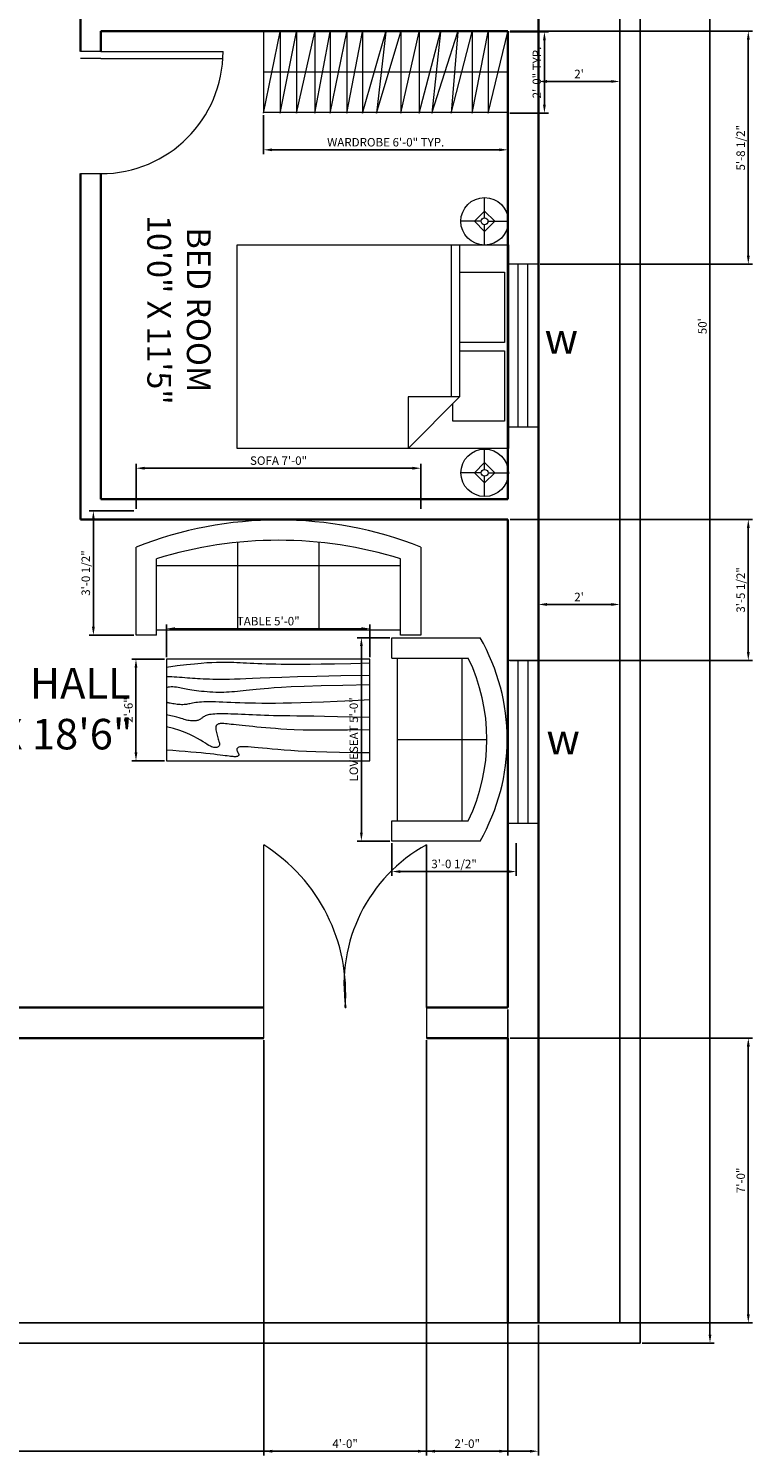
# Model space of a CAD drawing. Units: inches. Extents: x 1879 to 2382, y 1769 to 2461.
# Tile 3 of 5: x 2168 to 2382, y 1769 to 2190. Entities that reach past the tile are written whole.
import ezdxf

# ---------------------------------------------------------------- set-up
doc = ezdxf.new("R2010")
doc.units = ezdxf.units.IN
for name, color, linetype, lineweight in [('A-ANNO-DIMS', 2, 'Continuous', 18), ('A-ANNO-TEXT', 3, 'Continuous', 18), ('A-AREA-IDEN', 7, 'Continuous', 18), ('A-DOOR', 3, 'Continuous', 18), ('A-FLOR-CASE', 8, 'Continuous', 18), ('A-FURN', 9, 'Continuous', 18), ('A-GLAZ', 4, 'Continuous', 18), ('A-WALL', 7, 'Continuous', 35), ('C-PROP', 1, 'Continuous', 25)]:
    doc.layers.add(name, color=color, linetype=linetype, lineweight=lineweight)
doc.styles.get("Standard").update_dxf_attribs({"font": 'arial.ttf'})
doc.dimstyles.new('ISO-25', dxfattribs={"dimtxt": 2.5, "dimasz": 2.5, "dimexe": 1.25, "dimexo": 0.625, "dimtad": 1, "dimlunit": 4, "dimtxsty": 'Standard', "dimcen": 2.5, "dimadec": 0, "dimazin": 0, "dimtfac": 1, "dimtmove": 0, "dimatfit": 3, "dimfxl": 1, "dimarcsym": 0})

# ---------------------------------------------------------------- blocks, each defined once
blk = doc.blocks.new('*D2')
at = {"layer": 'A-ANNO-DIMS', "color": 0, "lineweight": -2, "transparency": 16777216}
for p, q in [((2348.97, 2402.18), (2370.19, 2402.18)), ((2368.94, 2399.68), (2368.94, 1804.68)), ((2348.97, 1802.18), (2370.19, 1802.18))]:
    blk.add_line(p, q, dxfattribs=at)
at = {"layer": 'A-ANNO-DIMS', "color": 0, "transparency": 16777216}
for points in [[(2368.53, 2399.68), (2369.36, 2399.68), (2368.94, 2402.18)], [(2368.53, 1804.68), (2369.36, 1804.68), (2368.94, 1802.18)]]:
    blk.add_solid(points, dxfattribs=at)
at = {"layer": 'Defpoints', "color": 0, "transparency": 16777216}
for p in [(2348.34, 2402.18), (2348.34, 1802.18), (2368.94, 1802.18)]:
    blk.add_point(p, dxfattribs=at)
at = {"layer": 'A-ANNO-DIMS', "color": 0, "transparency": 16777216, "insert": (2367.04, 2102.18), "char_height": 2.5, "attachment_point": 5, "rotation": 90}
blk.add_mtext("50'", dxfattribs=at)
blk = doc.blocks.new('Table - Rectangular Woodgrain 60 x 30 in.')
for p, q in [((0, 0), (0, -30)), ((60, 0), (0, 0)), ((60, -30), (60, 0)), ((0, -30), (60, -30))]:
    blk.add_line(p, q)
for points in [[(0, -2.4), (4.8155, -2.418), (9.0302, -2.4688), (12.709, -2.5477), (15.9167, -2.65), (18.7181, -2.7711), (21.1781, -2.9063), (23.3616, -3.0508), (25.3333, -3.2), (27.1477, -3.3495), (28.8172, -3.4958), (30.3437, -3.636), (31.7291, -3.7667), (32.9756, -3.8849), (34.0849, -3.9875), (35.059, -4.0714), (35.9, -4.1334), (36.6114, -4.1711), (37.2041, -4.1854), (37.6906, -4.1779), (38.0833, -4.15), (38.3948, -4.1034), (38.6375, -4.0396), (38.8239, -3.9602), (38.9666, -3.8667), (39.0764, -3.7608), (39.1573, -3.6448), (39.2116, -3.521), (39.2416, -3.3917), (39.2498, -3.2593), (39.2385, -3.1261), (39.21, -2.9944), (39.1666, -2.8667), (39.111, -2.7447), (39.0468, -2.6281), (38.978, -2.5163), (38.9083, -2.4083), (38.8418, -2.3035), (38.7823, -2.201), (38.7337, -2.1001), (38.7, -2), (38.6844, -1.9003), (38.6875, -1.8021), (38.7094, -1.707), (38.75, -1.6167), (38.8094, -1.5326), (38.8875, -1.4563), (38.9844, -1.3893), (39.1, -1.3333), (39.2351, -1.2896), (39.3937, -1.2583), (39.5804, -1.2396), (39.8, -1.2333), (40.057, -1.2396), (40.3562, -1.2583), (40.7023, -1.2896), (41.1, -1.3333), (41.5547, -1.3895), (42.0755, -1.4573), (42.6721, -1.5361), (43.3542, -1.625), (44.1316, -1.7233), (45.014, -1.8302), (46.0114, -1.9449), (47.1333, -2.0667), (48.3862, -2.1947), (49.7625, -2.3281), (51.2513, -2.4663), (52.8416, -2.6083), (54.5226, -2.7535), (56.2833, -2.9011), (58.1127, -3.0501), (60, -3.2)], [(0, -9.2), (6.5759, -9.0858), (11.9385, -9.0365), (16.2527, -9.0418), (19.6833, -9.0917), (22.3952, -9.1759), (24.5531, -9.2844), (26.322, -9.4069), (27.8666, -9.5333), (29.3241, -9.6553), (30.7203, -9.7719), (32.0532, -9.8837), (33.3208, -9.9917), (34.5213, -10.0965), (35.6526, -10.199), (36.7128, -10.2999), (37.7, -10.4), (38.6129, -10.4996), (39.4531, -10.5969), (40.223, -10.6895), (40.925, -10.775), (41.5613, -10.8512), (42.1344, -10.9156), (42.6465, -10.966), (43.1, -11), (43.4976, -11.0158), (43.8437, -11.0136), (44.143, -10.9942), (44.4, -10.9583), (44.6195, -10.9069), (44.8062, -10.8406), (44.9648, -10.7603), (45.1, -10.6667), (45.2155, -10.5598), (45.3114, -10.4365), (45.3871, -10.2929), (45.4416, -10.125), (45.4743, -9.929), (45.4844, -9.7011), (45.4709, -9.4371), (45.4333, -9.1333), (45.3716, -8.7883), (45.2896, -8.4104), (45.1919, -8.0107), (45.0833, -7.6), (44.9685, -7.1893), (44.8521, -6.7896), (44.7388, -6.4117), (44.6333, -6.0667), (44.54, -5.7628), (44.4614, -5.4979), (44.4001, -5.2675), (44.3583, -5.0667), (44.3384, -4.8909), (44.3427, -4.7354), (44.3736, -4.5956), (44.4333, -4.4667), (44.5236, -4.3453), (44.6427, -4.2333), (44.7884, -4.1339), (44.9583, -4.05), (45.1501, -3.9849), (45.3614, -3.9417), (45.59, -3.9234), (45.8333, -3.9333), (46.0915, -3.9749), (46.3734, -4.0531), (46.6906, -4.1736), (47.0542, -4.3417), (47.4756, -4.5629), (47.9661, -4.8427), (48.5372, -5.1866), (49.2, -5.6), (49.9676, -6.0844), (50.8594, -6.625), (51.8965, -7.2031), (53.1, -7.8), (54.491, -8.3969), (56.0906, -8.975), (57.9199, -9.5156), (60, -10)], [(0, -12.8), (5.1847, -12.9322), (9.6213, -13.0323), (13.3963, -13.1059), (16.5958, -13.1583), (19.3063, -13.1952), (21.614, -13.2219), (23.6054, -13.2439), (25.3666, -13.2667), (26.9728, -13.2947), (28.4531, -13.3281), (29.8256, -13.3663), (31.1083, -13.4083), (32.3191, -13.4535), (33.476, -13.501), (34.597, -13.5501), (35.7, -13.6), (36.7984, -13.6497), (37.8875, -13.6979), (38.9578, -13.743), (40, -13.7833), (41.0047, -13.8174), (41.9625, -13.8438), (42.864, -13.8607), (43.7, -13.8667), (44.4631, -13.8604), (45.1552, -13.8417), (45.7801, -13.8104), (46.3416, -13.7667), (46.8439, -13.7104), (47.2906, -13.6417), (47.6858, -13.5604), (48.0333, -13.4667), (48.3375, -13.3608), (48.6042, -13.2448), (48.8396, -13.121), (49.05, -12.9917), (49.2417, -12.8593), (49.4208, -12.7261), (49.5937, -12.5944), (49.7667, -12.4667), (49.9452, -12.3451), (50.1323, -12.2313), (50.3303, -12.1268), (50.5416, -12.0333), (50.7686, -11.9524), (51.0135, -11.8854), (51.2788, -11.8341), (51.5666, -11.8), (51.8785, -11.7843), (52.2116, -11.7865), (52.562, -11.8059), (52.926, -11.8417), (53.2998, -11.8931), (53.6795, -11.9594), (54.0614, -12.0397), (54.4416, -12.1333), (54.8223, -12.2401), (55.2293, -12.3625), (55.6942, -12.5037), (56.2489, -12.6667), (56.9251, -12.8547), (57.7545, -13.0708), (58.7689, -13.3182), (60, -13.6)], [(0, -18), (5.124, -17.7273), (9.6609, -17.5057), (13.6705, -17.3303), (17.2125, -17.1958), (20.3467, -17.0973), (23.1328, -17.0297), (25.6307, -16.9878), (27.9, -16.9667), (29.9928, -16.9617), (31.9302, -16.9703), (33.7254, -16.9907), (35.3917, -17.0208), (36.9423, -17.0588), (38.3906, -17.1026), (39.7499, -17.1503), (41.0333, -17.2), (42.2519, -17.2496), (43.4073, -17.2969), (44.4986, -17.3395), (45.525, -17.375), (46.4858, -17.4012), (47.3802, -17.4156), (48.2074, -17.416), (48.9667, -17.4), (49.6583, -17.3662), (50.2872, -17.3167), (50.8595, -17.2547), (51.3812, -17.1833), (51.8584, -17.1057), (52.2971, -17.025), (52.7034, -16.9443), (53.0833, -16.8667), (53.443, -16.7951), (53.789, -16.7313), (54.128, -16.6768), (54.4666, -16.6334), (54.8115, -16.6024), (55.1693, -16.5854), (55.5465, -16.5841), (55.95, -16.6), (56.3828, -16.6337), (56.8346, -16.6823), (57.2915, -16.7418), (57.7396, -16.8084), (58.165, -16.878), (58.5539, -16.9469), (58.8924, -17.0111), (59.1666, -17.0667), (59.3679, -17.1107), (59.5078, -17.1438), (59.6032, -17.1675), (59.6708, -17.1833), (59.7275, -17.193), (59.7901, -17.1979), (59.8753, -17.1998), (60, -17.2)], [(0, -22.4), (8.0098, -22.2501), (14.4094, -22.1011), (19.4168, -21.9535), (23.25, -21.8083), (26.1269, -21.6663), (28.2656, -21.5281), (29.884, -21.3947), (31.2, -21.2667), (32.3967, -21.1448), (33.5172, -21.0292), (34.5697, -20.9198), (35.5625, -20.8167), (36.5037, -20.7198), (37.4015, -20.6292), (38.2642, -20.5448), (39.1, -20.4667), (39.9164, -20.3951), (40.7187, -20.3313), (41.5117, -20.2768), (42.3, -20.2333), (43.0883, -20.2024), (43.8812, -20.1854), (44.6836, -20.1841), (45.5, -20.2), (46.3328, -20.234), (47.1747, -20.2844), (48.0163, -20.3488), (48.8479, -20.425), (49.66, -20.5106), (50.4429, -20.6031), (51.1872, -20.7004), (51.8833, -20.8), (52.5246, -20.8999), (53.1166, -20.9995), (53.6681, -21.0983), (54.1875, -21.1958), (54.6834, -21.2919), (55.1646, -21.3859), (55.6394, -21.4777), (56.1167, -21.5667), (56.6028, -21.6515), (57.0961, -21.7266), (57.5929, -21.7852), (58.0896, -21.8208), (58.5823, -21.8268), (59.0674, -21.7964), (59.5412, -21.723), (60, -21.6)], [(0, -25.2), (8.6355, -25.0504), (15.7026, -24.9031), (21.4049, -24.7606), (25.9458, -24.625), (29.529, -24.4988), (32.3578, -24.3844), (34.6359, -24.284), (36.5667, -24.2), (38.3213, -24.1341), (39.9417, -24.0854), (41.437, -24.0523), (42.8167, -24.0333), (44.0901, -24.0268), (45.2667, -24.0313), (46.3557, -24.0451), (47.3667, -24.0667), (48.309, -24.0947), (49.1928, -24.1287), (50.0284, -24.168), (50.826, -24.2125), (51.5959, -24.2617), (52.3483, -24.3151), (53.0935, -24.3725), (53.8417, -24.4334), (54.6009, -24.497), (55.3699, -24.561), (56.1454, -24.6226), (56.9239, -24.6792), (57.7021, -24.7279), (58.4764, -24.7662), (59.2435, -24.7911), (60, -24.8)], [(0, -28.8), (5.6867, -28.6681), (10.45, -28.5698), (14.407, -28.5012), (17.675, -28.4584), (20.3711, -28.4374), (22.6125, -28.4344), (24.5164, -28.4455), (26.2, -28.4667), (27.762, -28.4947), (29.2276, -28.5281), (30.6033, -28.5663), (31.8958, -28.6084), (33.1118, -28.6535), (34.2578, -28.7011), (35.3405, -28.7501), (36.3666, -28.8), (37.3443, -28.8497), (38.288, -28.8974), (39.2137, -28.9412), (40.1375, -28.9792), (41.0753, -29.0093), (42.0432, -29.0297), (43.0572, -29.0384), (44.1333, -29.0333), (45.2936, -29.0114), (46.5843, -28.9641), (48.0579, -28.8816), (49.7666, -28.7542), (51.7629, -28.5721), (54.0989, -28.3255), (56.8272, -28.0048), (60, -27.6)]]:
    blk.add_lwpolyline(points)
blk = doc.blocks.new('Sofa - Roundback 7 ft.')
for p, q in [((-12.00002, -32.4421), (-12.00003, -6.5971)), ((11.99997, -32.4421), (11.99998, -6.5971)), ((-36.000027, -34), (-36.000027, -11.4696)), ((35.99998, -34), (35.99998, -11.4696)), ((-35.999844, -13.3819), (35.9998, -13.3819)), ((-36.000027, -32.4421), (35.99998, -32.4421))]:
    blk.add_line(p, q)
for points in [[(-36.000027, -34), (-42.000027, -34), (-42.000027, -8)], [(41.99998, -8), (41.99998, -34), (35.99998, -34)]]:
    blk.add_lwpolyline(points)
for centre, radius, start, end in [((0, -114.25), 114.25, 68.43141, 111.5686), ((-0.00001, -127.1968), 121.1968, 72.72033, 107.2797)]:
    blk.add_arc(centre, radius, start, end)
blk = doc.blocks.new('Sofa - Roundback Loveseat 5 ft.')
for p, q in [((0, -32.44198), (0, -5.99998)), ((-24, -33.99998), (-24, -11.46958)), ((24.00004, -33.99998), (24.00004, -11.46958)), ((-23.9998, -13.38178), (23.99986, -13.38178)), ((-24, -32.44198), (24.00004, -32.44198))]:
    blk.add_line(p, q)
for points in [[(-24, -33.99998), (-30, -33.99998), (-30, -7.99998)], [(30.00004, -7.99998), (30.00004, -33.99998), (24.00004, -33.99998)]]:
    blk.add_lwpolyline(points)
for centre, radius, start, end in [((0, -60.24998), 60.24998, 60.13715, 119.8628), ((0, -61.38438), 55.38444, 64.32083, 115.6792)]:
    blk.add_arc(centre, radius, start, end)
blk = doc.blocks.new('Bed - Queen')
for p, q in [((0, -80.00003), (0, 0)), ((0, 0), (59.99999, 0)), ((59.99999, 0), (59.99999, -80.00003)), ((7.99999, -1.2), (28.79998, -1.2)), ((7.99999, -14.4), (7.99999, -1.2)), ((28.79998, -1.2), (28.79998, -14.4)), ((31.19999, -1.2), (51.99999, -1.2)), ((31.19999, -14.4), (31.19999, -1.2)), ((51.99999, -1.2), (51.99999, -16.4)), ((0, -14.4), (44.8, -14.4)), ((44.8, -16.8), (0, -16.8)), ((59.99999, -29.6), (44.8, -14.4)), ((44.8, -14.4), (44.8, -29.6)), ((51.99999, -16.4), (46.79936, -16.4)), ((44.8, -29.6), (59.99999, -29.6)), ((59.99999, -80.00003), (0, -80.00003))]:
    blk.add_line(p, q)
blk = doc.blocks.new('Lamp - Table')
for p, q in [((0, 7), (0, 1)), ((-1, 0), (-7, 0)), ((0, 3), (-3, 0)), ((-3, 0), (0, -3)), ((3, 0), (0, 3)), ((0, -3), (3, 0)), ((1, 0), (7, 0)), ((0, -1), (0, -7))]:
    blk.add_line(p, q)
for radius in [7, 1]:
    blk.add_circle((0, 0), radius)
blk = doc.blocks.new('*D17')
at = {"layer": 'A-ANNO-DIMS', "color": 0, "lineweight": -2, "transparency": 16777216}
for p, q in [((2318.34, 2188.56), (2318.34, 2173.13)), ((2342.34, 2188.56), (2342.34, 2173.13)), ((2320.84, 2174.38), (2339.84, 2174.38))]:
    blk.add_line(p, q, dxfattribs=at)
at = {"layer": 'A-ANNO-DIMS', "color": 0, "transparency": 16777216}
for points in [[(2320.84, 2174.8), (2320.84, 2173.97), (2318.34, 2174.38)], [(2339.84, 2174.8), (2339.84, 2173.97), (2342.34, 2174.38)]]:
    blk.add_solid(points, dxfattribs=at)
at = {"layer": 'Defpoints', "color": 0, "transparency": 16777216}
for p in [(2318.34, 2189.18), (2342.34, 2189.18), (2342.34, 2174.38)]:
    blk.add_point(p, dxfattribs=at)
at = {"layer": 'A-ANNO-DIMS', "color": 0, "transparency": 16777216, "insert": (2330.34, 2176.26), "char_height": 2.5, "attachment_point": 5}
blk.add_mtext("2'", dxfattribs=at)
blk = doc.blocks.new('*D18')
at = {"layer": 'A-ANNO-DIMS', "color": 0, "lineweight": -2, "transparency": 16777216}
for p, q in [((2318.34, 2020.71), (2318.34, 2021.34)), ((2342.34, 2020.71), (2342.34, 2021.34)), ((2339.84, 2020.09), (2320.84, 2020.09))]:
    blk.add_line(p, q, dxfattribs=at)
at = {"layer": 'A-ANNO-DIMS', "color": 0, "transparency": 16777216}
for points in [[(2320.84, 2020.51), (2320.84, 2019.67), (2318.34, 2020.09)], [(2339.84, 2020.51), (2339.84, 2019.67), (2342.34, 2020.09)]]:
    blk.add_solid(points, dxfattribs=at)
at = {"layer": 'Defpoints', "color": 0, "transparency": 16777216}
for p in [(2318.34, 2020.09), (2318.34, 2020.09), (2342.34, 2020.09)]:
    blk.add_point(p, dxfattribs=at)
at = {"layer": 'A-ANNO-DIMS', "color": 0, "transparency": 16777216, "insert": (2330.34, 2021.97), "char_height": 2.5, "attachment_point": 5}
blk.add_mtext("2'", dxfattribs=at)
blk = doc.blocks.new('WN-48x9')
for p, q in [((0, 48), (0, 0)), ((9, 48), (0, 48)), ((3, 48), (3, 0)), ((6, 0), (6, 48)), ((9, 0), (9, 48)), ((0, 0), (9, 0))]:
    blk.add_line(p, q)
blk = doc.blocks.new('DR-SWING-36')
for p, q in [((42, 36), (36, 36)), ((36, 2), (0, 2)), ((36, 0), (0, 0)), ((36, 2), (42, 2)), ((36, 0), (42, 0))]:
    blk.add_line(p, q)
blk.add_arc((36, 0), 36, 90, 180)
blk = doc.blocks.new('WARDROBE-HANGERS-72')
for p, q in [((0, 0), (4.89, 24)), ((4.89, 24), (4.89, 0)), ((4.89, 0), (9.67, 24)), ((9.67, 24), (9.67, 0)), ((9.67, 0), (15.08, 24)), ((15.08, 24), (15.08, 0)), ((15.08, 0), (19.6, 24)), ((19.6, 24), (19.6, 0)), ((19.6, 0), (24.51, 24)), ((24.51, 24), (24.51, 0)), ((24.51, 0), (29.16, 24)), ((29.16, 24), (29.16, 0)), ((29.16, 0), (36, 24)), ((36, 24), (33.31, 0)), ((33.31, 0), (40.47, 24)), ((40.47, 24), (40.47, 0)), ((40.47, 0), (45.88, 24)), ((45.88, 24), (45.88, 0)), ((45.88, 0), (52.17, 24)), ((52.17, 24), (49.65, 0)), ((49.65, 0), (57.32, 24)), ((57.32, 24), (55.31, 0)), ((55.31, 0), (61.47, 24)), ((61.47, 24), (61.47, 0)), ((61.47, 0), (66.25, 24)), ((66.25, 24), (66.25, 0)), ((66.25, 0), (72, 24))]:
    blk.add_line(p, q)
blk = doc.blocks.new('*D37')
at = {"layer": 'A-ANNO-DIMS', "color": 0, "lineweight": -2, "transparency": 16777216}
for p, q in [((2237.31, 2164.39), (2237.31, 2152.97)), ((2309.31, 2164.39), (2309.31, 2152.97)), ((2239.81, 2154.22), (2306.81, 2154.22))]:
    blk.add_line(p, q, dxfattribs=at)
at = {"layer": 'A-ANNO-DIMS', "color": 0, "transparency": 16777216}
for points in [[(2239.81, 2154.63), (2239.81, 2153.8), (2237.31, 2154.22)], [(2306.81, 2154.63), (2306.81, 2153.8), (2309.31, 2154.22)]]:
    blk.add_solid(points, dxfattribs=at)
at = {"layer": 'Defpoints', "color": 0, "transparency": 16777216}
for p in [(2237.31, 2165.02), (2309.31, 2165.02), (2309.31, 2154.22)]:
    blk.add_point(p, dxfattribs=at)
at = {"layer": 'A-ANNO-DIMS', "color": 0, "transparency": 16777216, "insert": (2273.31, 2156.13), "char_height": 2.5, "attachment_point": 5}
blk.add_mtext('WARDROBE 6\'-0" TYP.', dxfattribs=at)
blk = doc.blocks.new('*D38')
at = {"layer": 'A-ANNO-DIMS', "color": 0, "lineweight": -2, "transparency": 16777216}
for p, q in [((2309.93, 2189.02), (2321.36, 2189.02)), ((2320.11, 2167.52), (2320.11, 2186.52)), ((2309.93, 2165.02), (2321.36, 2165.02))]:
    blk.add_line(p, q, dxfattribs=at)
at = {"layer": 'A-ANNO-DIMS', "color": 0, "transparency": 16777216}
for points in [[(2319.69, 2186.52), (2320.53, 2186.52), (2320.11, 2189.02)], [(2319.69, 2167.52), (2320.53, 2167.52), (2320.11, 2165.02)]]:
    blk.add_solid(points, dxfattribs=at)
at = {"layer": 'Defpoints', "color": 0, "transparency": 16777216}
for p in [(2309.31, 2189.02), (2320.11, 2189.02), (2309.31, 2165.02)]:
    blk.add_point(p, dxfattribs=at)
at = {"layer": 'A-ANNO-DIMS', "color": 0, "transparency": 16777216, "insert": (2318.21, 2177.02), "char_height": 2.5, "attachment_point": 5, "rotation": 90}
blk.add_mtext('2\'-0" TYP.', dxfattribs=at)
blk = doc.blocks.new('*D47')
at = {"layer": 'A-ANNO-DIMS', "color": 0, "lineweight": -2, "transparency": 16777216}
for p, q in [((2199.71, 2048.3), (2199.71, 2061.53)), ((2202.21, 2060.28), (2281.21, 2060.28)), ((2283.71, 2048.3), (2283.71, 2061.53))]:
    blk.add_line(p, q, dxfattribs=at)
at = {"layer": 'A-ANNO-DIMS', "color": 0, "transparency": 16777216}
for points in [[(2202.21, 2060.7), (2202.21, 2059.86), (2199.71, 2060.28)], [(2281.21, 2060.7), (2281.21, 2059.86), (2283.71, 2060.28)]]:
    blk.add_solid(points, dxfattribs=at)
at = {"layer": 'Defpoints', "color": 0, "transparency": 16777216}
for p in [(2283.71, 2060.28), (2199.71, 2047.68), (2283.71, 2047.68)]:
    blk.add_point(p, dxfattribs=at)
at = {"layer": 'A-ANNO-DIMS', "color": 0, "transparency": 16777216, "insert": (2241.71, 2062.2), "char_height": 2.5, "attachment_point": 5}
blk.add_mtext('SOFA 7\'-0"', dxfattribs=at)
blk = doc.blocks.new('*D48')
at = {"layer": 'A-ANNO-DIMS', "color": 0, "lineweight": -2, "transparency": 16777216}
for p, q in [((2199.08, 2047.68), (2185.86, 2047.68)), ((2187.11, 2013.51), (2187.11, 2045.18)), ((2199.08, 2011.01), (2185.86, 2011.01))]:
    blk.add_line(p, q, dxfattribs=at)
at = {"layer": 'A-ANNO-DIMS', "color": 0, "transparency": 16777216}
for points in [[(2186.69, 2045.18), (2187.52, 2045.18), (2187.11, 2047.68)], [(2186.69, 2013.51), (2187.52, 2013.51), (2187.11, 2011.01)]]:
    blk.add_solid(points, dxfattribs=at)
at = {"layer": 'Defpoints', "color": 0, "transparency": 16777216}
for p in [(2187.11, 2047.68), (2199.71, 2047.68), (2199.71, 2011.01)]:
    blk.add_point(p, dxfattribs=at)
at = {"layer": 'A-ANNO-DIMS', "color": 0, "transparency": 16777216, "insert": (2185.19, 2029.35), "char_height": 2.5, "attachment_point": 5, "rotation": 90}
blk.add_mtext('3\'-0 1/2"', dxfattribs=at)
blk = doc.blocks.new('*D49')
at = {"layer": 'A-ANNO-DIMS', "color": 0, "lineweight": -2, "transparency": 16777216}
for p, q in [((2274.52, 2010.29), (2264.89, 2010.29)), ((2266.14, 2007.79), (2266.14, 1952.79)), ((2274.52, 1950.29), (2264.89, 1950.29))]:
    blk.add_line(p, q, dxfattribs=at)
at = {"layer": 'A-ANNO-DIMS', "color": 0, "transparency": 16777216}
for points in [[(2265.73, 2007.79), (2266.56, 2007.79), (2266.14, 2010.29)], [(2265.73, 1952.79), (2266.56, 1952.79), (2266.14, 1950.29)]]:
    blk.add_solid(points, dxfattribs=at)
at = {"layer": 'Defpoints', "color": 0, "transparency": 16777216}
for p in [(2275.14, 2010.29), (2266.14, 1950.29), (2275.14, 1950.29)]:
    blk.add_point(p, dxfattribs=at)
at = {"layer": 'A-ANNO-DIMS', "color": 0, "transparency": 16777216, "insert": (2264.22, 1980.29), "char_height": 2.5, "attachment_point": 5, "rotation": 90}
blk.add_mtext('LOVESEAT 5\'-0"', dxfattribs=at)
blk = doc.blocks.new('*D50')
at = {"layer": 'A-ANNO-DIMS', "color": 0, "lineweight": -2, "transparency": 16777216}
for p, q in [((2275.14, 1949.66), (2275.14, 1940.04)), ((2311.81, 1949.66), (2311.81, 1940.04)), ((2277.64, 1941.29), (2309.31, 1941.29))]:
    blk.add_line(p, q, dxfattribs=at)
at = {"layer": 'A-ANNO-DIMS', "color": 0, "transparency": 16777216}
for points in [[(2277.64, 1941.7), (2277.64, 1940.87), (2275.14, 1941.29)], [(2309.31, 1941.7), (2309.31, 1940.87), (2311.81, 1941.29)]]:
    blk.add_solid(points, dxfattribs=at)
at = {"layer": 'Defpoints', "color": 0, "transparency": 16777216}
for p in [(2275.14, 1950.29), (2311.81, 1950.29), (2311.81, 1941.29)]:
    blk.add_point(p, dxfattribs=at)
at = {"layer": 'A-ANNO-DIMS', "color": 0, "transparency": 16777216, "insert": (2293.48, 1943.21), "char_height": 2.5, "attachment_point": 5}
blk.add_mtext('3\'-0 1/2"', dxfattribs=at)
blk = doc.blocks.new('*D51')
at = {"layer": 'A-ANNO-DIMS', "color": 0, "lineweight": -2, "transparency": 16777216}
for p, q in [((2208.67, 2004.57), (2208.67, 2014.19)), ((2266.17, 2012.94), (2211.17, 2012.94)), ((2268.67, 2004.57), (2268.67, 2014.19))]:
    blk.add_line(p, q, dxfattribs=at)
at = {"layer": 'A-ANNO-DIMS', "color": 0, "transparency": 16777216}
for points in [[(2211.17, 2013.36), (2211.17, 2012.52), (2208.67, 2012.94)], [(2266.17, 2013.36), (2266.17, 2012.52), (2268.67, 2012.94)]]:
    blk.add_solid(points, dxfattribs=at)
at = {"layer": 'Defpoints', "color": 0, "transparency": 16777216}
for p in [(2208.67, 2012.94), (2208.67, 2003.94), (2268.67, 2003.94)]:
    blk.add_point(p, dxfattribs=at)
at = {"layer": 'A-ANNO-DIMS', "color": 0, "transparency": 16777216, "insert": (2238.67, 2014.84), "char_height": 2.5, "attachment_point": 5}
blk.add_mtext('TABLE 5\'-0"', dxfattribs=at)
blk = doc.blocks.new('*D52')
at = {"layer": 'A-ANNO-DIMS', "color": 0, "lineweight": -2, "transparency": 16777216}
for p, q in [((2208.04, 2003.94), (2198.42, 2003.94)), ((2199.67, 2001.44), (2199.67, 1976.44)), ((2208.04, 1973.94), (2198.42, 1973.94))]:
    blk.add_line(p, q, dxfattribs=at)
at = {"layer": 'A-ANNO-DIMS', "color": 0, "transparency": 16777216}
for points in [[(2199.25, 2001.44), (2200.08, 2001.44), (2199.67, 2003.94)], [(2199.25, 1976.44), (2200.08, 1976.44), (2199.67, 1973.94)]]:
    blk.add_solid(points, dxfattribs=at)
at = {"layer": 'Defpoints', "color": 0, "transparency": 16777216}
for p in [(2208.67, 2003.94), (2199.67, 1973.94), (2208.67, 1973.94)]:
    blk.add_point(p, dxfattribs=at)
at = {"layer": 'A-ANNO-DIMS', "color": 0, "transparency": 16777216, "insert": (2197.77, 1988.94), "char_height": 2.5, "attachment_point": 5, "rotation": 90}
blk.add_mtext('2\'-6"', dxfattribs=at)
blk = doc.blocks.new('*D55')
at = {"layer": 'A-ANNO-DIMS', "color": 0, "lineweight": -2, "transparency": 16777216}
for p, q in [((1946.34, 1807.56), (1946.34, 1769.03)), ((2318.34, 1807.56), (2318.34, 1769.03)), ((1948.84, 1770.28), (2315.84, 1770.28))]:
    blk.add_line(p, q, dxfattribs=at)
at = {"layer": 'A-ANNO-DIMS', "color": 0, "transparency": 16777216}
for points in [[(1948.84, 1770.7), (1948.84, 1769.86), (1946.34, 1770.28)], [(2315.84, 1770.7), (2315.84, 1769.86), (2318.34, 1770.28)]]:
    blk.add_solid(points, dxfattribs=at)
at = {"layer": 'Defpoints', "color": 0, "transparency": 16777216}
for p in [(1946.34, 1808.18), (2318.34, 1808.18), (2318.34, 1770.28)]:
    blk.add_point(p, dxfattribs=at)
at = {"layer": 'A-ANNO-DIMS', "color": 0, "transparency": 16777216, "insert": (2132.34, 1772.18), "char_height": 2.5, "attachment_point": 5}
blk.add_mtext('31\'-0"', dxfattribs=at)
blk = doc.blocks.new('*D57')
at = {"layer": 'A-ANNO-DIMS', "color": 0, "lineweight": -2, "transparency": 16777216}
for p, q in [((2309.97, 1892.18), (2381.49, 1892.18)), ((2380.24, 1889.68), (2380.24, 1810.68)), ((2309.97, 1808.18), (2381.49, 1808.18))]:
    blk.add_line(p, q, dxfattribs=at)
at = {"layer": 'A-ANNO-DIMS', "color": 0, "transparency": 16777216}
for points in [[(2379.82, 1889.68), (2380.66, 1889.68), (2380.24, 1892.18)], [(2379.82, 1810.68), (2380.66, 1810.68), (2380.24, 1808.18)]]:
    blk.add_solid(points, dxfattribs=at)
at = {"layer": 'Defpoints', "color": 0, "transparency": 16777216}
for p in [(2309.34, 1892.18), (2309.34, 1808.18), (2380.24, 1808.18)]:
    blk.add_point(p, dxfattribs=at)
at = {"layer": 'A-ANNO-DIMS', "color": 0, "transparency": 16777216, "insert": (2378.34, 1850.18), "char_height": 2.5, "attachment_point": 5, "rotation": 90}
blk.add_mtext('7\'-0"', dxfattribs=at)
blk = doc.blocks.new('*D59')
at = {"layer": 'A-ANNO-DIMS', "color": 0, "lineweight": -2, "transparency": 16777216}
for p, q in [((2237.34, 1891.56), (2237.34, 1769.03)), ((2285.34, 1891.56), (2285.34, 1769.03)), ((2239.84, 1770.28), (2282.84, 1770.28))]:
    blk.add_line(p, q, dxfattribs=at)
at = {"layer": 'A-ANNO-DIMS', "color": 0, "transparency": 16777216}
for points in [[(2239.84, 1770.7), (2239.84, 1769.86), (2237.34, 1770.28)], [(2282.84, 1770.7), (2282.84, 1769.86), (2285.34, 1770.28)]]:
    blk.add_solid(points, dxfattribs=at)
at = {"layer": 'Defpoints', "color": 0, "transparency": 16777216}
for p in [(2237.34, 1892.18), (2285.34, 1892.18), (2285.34, 1770.28)]:
    blk.add_point(p, dxfattribs=at)
at = {"layer": 'A-ANNO-DIMS', "color": 0, "transparency": 16777216, "insert": (2261.34, 1772.18), "char_height": 2.5, "attachment_point": 5}
blk.add_mtext('4\'-0"', dxfattribs=at)
blk = doc.blocks.new('*D60')
at = {"layer": 'A-ANNO-DIMS', "color": 0, "lineweight": -2, "transparency": 16777216}
for p, q in [((2309.34, 1900.56), (2309.34, 1769.03)), ((2285.34, 1891.56), (2285.34, 1769.03)), ((2287.84, 1770.28), (2306.84, 1770.28))]:
    blk.add_line(p, q, dxfattribs=at)
at = {"layer": 'A-ANNO-DIMS', "color": 0, "transparency": 16777216}
for points in [[(2287.84, 1770.7), (2287.84, 1769.86), (2285.34, 1770.28)], [(2306.84, 1770.7), (2306.84, 1769.86), (2309.34, 1770.28)]]:
    blk.add_solid(points, dxfattribs=at)
at = {"layer": 'Defpoints', "color": 0, "transparency": 16777216}
for p in [(2309.34, 1901.18), (2285.34, 1892.18), (2309.34, 1770.28)]:
    blk.add_point(p, dxfattribs=at)
at = {"layer": 'A-ANNO-DIMS', "color": 0, "transparency": 16777216, "insert": (2297.34, 1772.18), "char_height": 2.5, "attachment_point": 5}
blk.add_mtext('2\'-0"', dxfattribs=at)
blk = doc.blocks.new('*D69')
at = {"layer": 'A-ANNO-DIMS', "color": 0, "lineweight": -2, "transparency": 16777216}
for p, q in [((2309.97, 2189.18), (2381.49, 2189.18)), ((2380.24, 2122.96), (2380.24, 2186.68)), ((2318.89, 2120.46), (2381.49, 2120.46))]:
    blk.add_line(p, q, dxfattribs=at)
at = {"layer": 'A-ANNO-DIMS', "color": 0, "transparency": 16777216}
for points in [[(2379.82, 2186.68), (2380.66, 2186.68), (2380.24, 2189.18)], [(2379.82, 2122.96), (2380.66, 2122.96), (2380.24, 2120.46)]]:
    blk.add_solid(points, dxfattribs=at)
at = {"layer": 'Defpoints', "color": 0, "transparency": 16777216}
for p in [(2309.34, 2189.18), (2380.24, 2189.18), (2318.27, 2120.46)]:
    blk.add_point(p, dxfattribs=at)
at = {"layer": 'A-ANNO-DIMS', "color": 0, "transparency": 16777216, "insert": (2378.32, 2154.82), "char_height": 2.5, "attachment_point": 5, "rotation": 90}
blk.add_mtext('5\'-8 1/2"', dxfattribs=at)
blk = doc.blocks.new('*D76')
at = {"layer": 'A-ANNO-DIMS', "color": 0, "lineweight": -2, "transparency": 16777216}
for p, q in [((2309.97, 2045.18), (2381.49, 2045.18)), ((2380.24, 2042.68), (2380.24, 2006.07)), ((2309.94, 2003.57), (2381.49, 2003.57))]:
    blk.add_line(p, q, dxfattribs=at)
at = {"layer": 'A-ANNO-DIMS', "color": 0, "transparency": 16777216}
for points in [[(2379.82, 2042.68), (2380.66, 2042.68), (2380.24, 2045.18)], [(2379.82, 2006.07), (2380.66, 2006.07), (2380.24, 2003.57)]]:
    blk.add_solid(points, dxfattribs=at)
at = {"layer": 'Defpoints', "color": 0, "transparency": 16777216}
for p in [(2309.34, 2045.18), (2309.31, 2003.57), (2380.24, 2003.57)]:
    blk.add_point(p, dxfattribs=at)
at = {"layer": 'A-ANNO-DIMS', "color": 0, "transparency": 16777216, "insert": (2378.32, 2024.38), "char_height": 2.5, "attachment_point": 5, "rotation": 90}
blk.add_mtext('3\'-5 1/2"', dxfattribs=at)

msp = doc.modelspace()

# ---------------------------------------------------------------- linework, layer by layer
at = {"layer": 'A-DOOR'}
for p, q in [((2237.341, 1901.18), (2237.341, 1949.18)), ((2285.341, 1901.18), (2285.341, 1949.18)), ((2285.341, 1949.18), (2285.341, 1901.18)), ((2237.341, 1892.18), (2237.341, 1901.18)), ((2261.341, 1901.18), (2261.507, 1901.18)), ((2261.507, 1901.18), (2261.341, 1901.18)), ((2261.507, 1901.18), (2261.341, 1901.18)), ((2285.341, 1901.18), (2285.341, 1892.18))]:
    msp.add_line(p, q, dxfattribs=at)
for centre, radius, start, end in [((2209.623, 1905.321), 51.883, 355.42213, 57.70797), ((2307.924, 1908.049), 46.923, 118.76884, 188.41761)]:
    msp.add_arc(centre, radius, start, end, dxfattribs=at)
at = {"layer": 'A-FLOR-CASE'}
for p, q in [((2237.341, 2165.18), (2237.341, 2189.18)), ((2309.341, 2189.18), (2309.341, 2165.18)), ((2237.341, 2177.18), (2309.341, 2177.18)), ((2309.341, 2165.18), (2237.341, 2165.18))]:
    msp.add_line(p, q, dxfattribs=at)
at = {"layer": 'A-WALL'}
for p, q in [((2318.341, 2369.18), (2318.341, 1808.18)), ((2183.341, 2205.18), (2183.341, 2189.18)), ((2183.341, 2189.18), (2183.341, 2183.18)), ((2189.341, 2189.18), (2309.341, 2189.18)), ((2189.341, 2189.18), (2189.341, 2183.18)), ((2189.341, 2189.18), (2189.341, 2183.18)), ((2309.341, 2189.18), (2309.341, 2051.18)), ((2183.341, 2147.18), (2183.341, 2045.18)), ((2189.341, 2147.18), (2189.341, 2051.18)), ((2189.341, 2051.18), (2309.341, 2051.18)), ((2183.341, 2045.18), (2309.341, 2045.18)), ((2309.341, 2045.18), (2309.341, 1901.18)), ((2237.341, 1901.18), (2150.341, 1901.18)), ((2309.341, 1901.18), (2285.341, 1901.18)), ((2309.341, 1901.18), (2285.341, 1901.18)), ((2237.341, 1892.18), (1955.341, 1892.18)), ((2309.341, 1892.18), (2285.341, 1892.18)), ((2309.341, 1892.18), (2309.341, 1808.18))]:
    msp.add_line(p, q, dxfattribs=at)
at = {"layer": 'C-PROP'}
for p, q in [((2348.341, 2402.18), (2348.341, 1802.18)), ((2342.341, 2396.18), (2342.341, 1808.18)), ((2342.341, 1808.18), (1922.341, 1808.18)), ((2348.341, 1802.18), (1916.341, 1802.18))]:
    msp.add_line(p, q, dxfattribs=at)

# ---------------------------------------------------------------- block references
at = {"layer": 'A-DOOR', "rotation": 180}
msp.add_blockref('DR-SWING-36', (2225.341, 2183.18), dxfattribs=at)
at = {"layer": 'A-FLOR-CASE'}
msp.add_blockref('WARDROBE-HANGERS-72', (2237.308, 2165.016), dxfattribs=at)
at = {"layer": 'A-FURN'}
for name, p, rotation in [('Lamp - Table', (2302.467, 2133.133), 180), ('Bed - Queen', (2309.514, 2126.141), 270), ('Lamp - Table', (2302.48, 2058.931), 180), ('Sofa - Roundback Loveseat 5 ft.', (2309.143, 1980.287), 270), ('Table - Rectangular Woodgrain 60 x 30 in.', (2268.667, 1973.94), 180)]:
    msp.add_blockref(name, p, dxfattribs=dict(at, rotation=rotation))
msp.add_blockref('Sofa - Roundback 7 ft.', (2241.708, 2045.013), dxfattribs=at)
at = {"layer": 'A-GLAZ', "rotation": 180}
for p in [(2318.269, 2120.462), (2318.314, 2003.571)]:
    msp.add_blockref('WN-48x9', p, dxfattribs=at)

# ---------------------------------------------------------------- texts
at = {"layer": 'A-ANNO-TEXT', "char_height": 9, "attachment_point": 1}
for insert in [(2268.982, 2103.072), (2269.515, 1984.882)]:
    msp.add_mtext_dynamic_manual_height_columns('\\pxqc;w', width=112.22887, gutter_width=12.5, heights=[0], dxfattribs=dict(at, insert=insert))
at = {"layer": 'A-AREA-IDEN', "insert": (2221.675, 2153.078), "char_height": 7, "attachment_point": 1, "rotation": 270}
msp.add_mtext_dynamic_manual_height_columns('\\pxqc;BED ROOM\\P10\'0" X 11\'5"', width=92.15185, gutter_width=12.5, heights=[0], dxfattribs=at)
at = {"layer": 'A-AREA-IDEN', "insert": (2119.688, 2001.337), "char_height": 9, "attachment_point": 1}
msp.add_mtext_dynamic_manual_height_columns('\\pxqc;LIVING HALL\\P12\'0" X 18\'6"', width=86.0711, gutter_width=12.5, heights=[0], dxfattribs=at)

# ---------------------------------------------------------------- dimensions: what is measured, and where the dimension line sits
at = {"layer": 'A-ANNO-DIMS'}
for base, p1, p2, angle, override, picture, middle in [((2368.943, 1802.18), (2348.341, 2402.18), (2348.341, 1802.18), 90, {"dimclrd": 0, "dimclre": 0, "dimclrt": 0}, '*D2', (2367.042, 2102.18)), ((2380.241, 2189.18), (2318.269, 2120.462), (2309.341, 2189.18), 90, {"dimdec": 1, "dimlfac": 1, "dimrnd": 0, "dimzin": 1, "dimdsep": 46, "dimlunit": 4, "dimfrac": 2}, '*D69', (2378.324, 2154.821)), ((2187.108, 2047.68), (2199.708, 2011.013), (2199.708, 2047.68), 90, {"dimdec": 1, "dimlfac": 1, "dimrnd": 0, "dimzin": 1, "dimdsep": 46, "dimlunit": 4, "dimfrac": 2}, '*D48', (2185.189, 2029.346)), ((2380.241, 2003.571), (2309.341, 2045.18), (2309.314, 2003.571), 90, {"dimdec": 1, "dimlfac": 1, "dimrnd": 0, "dimzin": 1, "dimdsep": 46, "dimlunit": 4, "dimfrac": 2}, '*D76', (2378.323, 2024.376)), ((2199.667, 1973.94), (2208.667, 2003.94), (2208.667, 1973.94), 270, {"dimdec": 1, "dimlfac": 1, "dimrnd": 0, "dimzin": 1, "dimdsep": 46, "dimlunit": 4, "dimfrac": 2}, '*D52', (2197.766, 1988.94)), ((2380.241, 1808.18), (2309.341, 1892.18), (2309.341, 1808.18), 90, {"dimdec": 1, "dimlfac": 1, "dimrnd": 0, "dimzin": 1, "dimdsep": 46, "dimlunit": 4, "dimfrac": 2}, '*D57', (2378.34, 1850.18))]:
    dim = msp.add_linear_dim(base=base, p1=p1, p2=p2, angle=angle, dimstyle='ISO-25', override=override, dxfattribs=at)
    dim.commit()
    dim.dimension.update_dxf_attribs({"geometry": picture, "text_midpoint": middle})
for base, p1, p2, angle, text, picture, middle in [((2320.108, 2189.016), (2309.308, 2165.016), (2309.308, 2189.016), 90, '<> TYP.', '*D38', (2318.207, 2177.016)), ((2208.667, 2012.94), (2268.667, 2003.94), (2208.667, 2003.94), 180, 'TABLE <>', '*D51', (2238.667, 2014.842)), ((2266.143, 1950.287), (2275.143, 2010.287), (2275.143, 1950.287), 270, 'LOVESEAT <>', '*D49', (2264.225, 1980.287))]:
    dim = msp.add_linear_dim(base=base, p1=p1, p2=p2, angle=angle, text=text, dimstyle='ISO-25', override={"dimdec": 1, "dimlfac": 1, "dimrnd": 0, "dimzin": 1, "dimdsep": 46, "dimlunit": 4, "dimfrac": 2}, dxfattribs=at)
    dim.commit()
    dim.dimension.update_dxf_attribs({"geometry": picture, "text_midpoint": middle})
for base, p1, p2, override, picture, middle in [((2342.341, 2174.384), (2318.341, 2189.18), (2342.341, 2189.18), {"dimclrd": 0, "dimclre": 0, "dimclrt": 0}, '*D17', (2330.341, 2176.264)), ((2318.341, 2020.089), (2342.341, 2020.089), (2318.341, 2020.089), {"dimclrd": 0, "dimclre": 0, "dimclrt": 0}, '*D18', (2330.341, 2021.969)), ((2311.81, 1941.287), (2275.143, 1950.287), (2311.81, 1950.287), {"dimdec": 1, "dimlfac": 1, "dimrnd": 0, "dimzin": 1, "dimdsep": 46, "dimlunit": 4, "dimfrac": 2}, '*D50', (2293.477, 1943.205)), ((2309.341, 1770.28), (2285.341, 1892.18), (2309.341, 1901.18), {"dimdec": 1, "dimlfac": 1, "dimrnd": 0, "dimzin": 1, "dimdsep": 46, "dimlunit": 4, "dimfrac": 2}, '*D60', (2297.341, 1772.182)), ((2285.341, 1770.28), (2237.341, 1892.18), (2285.341, 1892.18), {"dimdec": 1, "dimlfac": 1, "dimrnd": 0, "dimzin": 1, "dimdsep": 46, "dimlunit": 4, "dimfrac": 2}, '*D59', (2261.341, 1772.182)), ((2318.341, 1770.28), (1946.341, 1808.18), (2318.341, 1808.18), {"dimdec": 1, "dimlfac": 1, "dimrnd": 0, "dimzin": 1, "dimdsep": 46, "dimlunit": 4, "dimfrac": 2}, '*D55', (2132.341, 1772.183))]:
    dim = msp.add_linear_dim(base=base, p1=p1, p2=p2, dimstyle='ISO-25', override=override, dxfattribs=at)
    dim.commit()
    dim.dimension.update_dxf_attribs({"geometry": picture, "text_midpoint": middle})
for base, p1, p2, text, picture, middle in [((2309.308, 2154.216), (2237.308, 2165.016), (2309.308, 2165.016), 'WARDROBE <> TYP.', '*D37', (2273.308, 2156.135)), ((2283.708, 2060.28), (2199.708, 2047.68), (2283.708, 2047.68), 'SOFA <>', '*D47', (2241.708, 2062.198))]:
    dim = msp.add_linear_dim(base=base, p1=p1, p2=p2, text=text, dimstyle='ISO-25', override={"dimdec": 1, "dimlfac": 1, "dimrnd": 0, "dimzin": 1, "dimdsep": 46, "dimlunit": 4, "dimfrac": 2}, dxfattribs=at)
    dim.commit()
    dim.dimension.update_dxf_attribs({"geometry": picture, "text_midpoint": middle})

doc.saveas('drawing.dxf')
